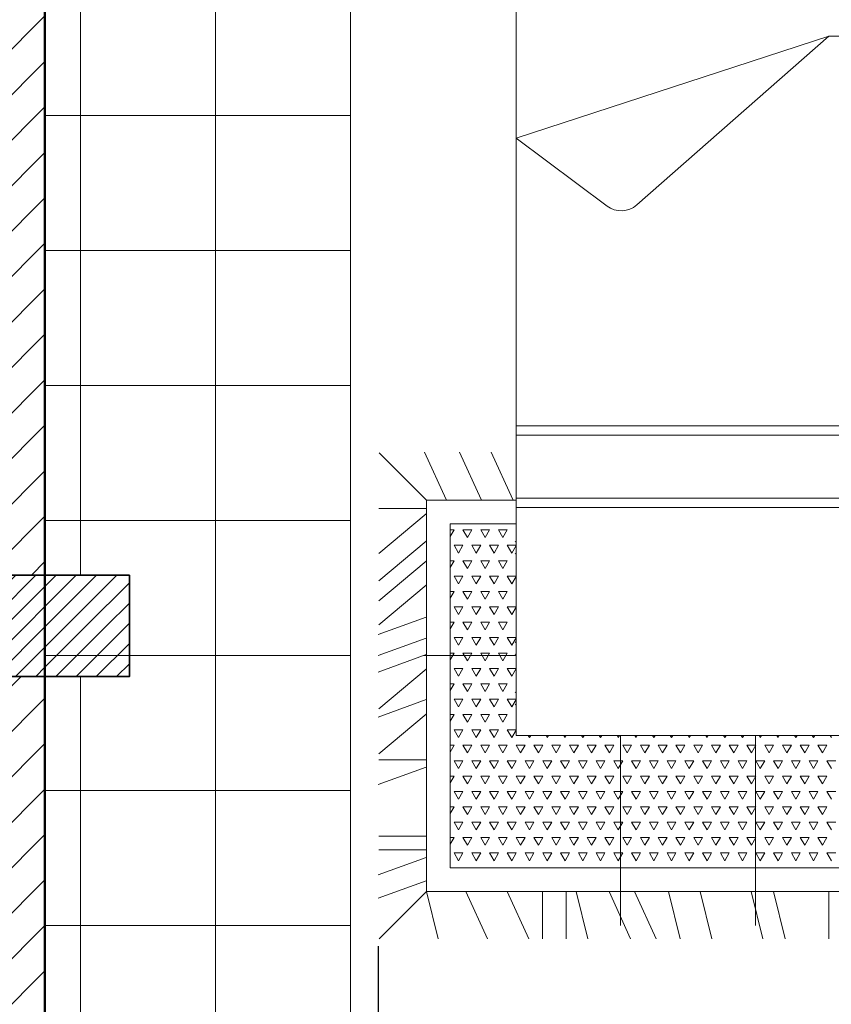
# Model space of a CAD drawing. Units: millimetres. Extents: x 225995 to 227247, y 225507 to 226008.
# Tile 19 of 23: x 227029 to 227101, y 225781 to 225868. Entities that reach past the tile are written whole.
import ezdxf

# ---------------------------------------------------------------- set-up
doc = ezdxf.new("R2010")
doc.units = ezdxf.units.MM
for name, color, linetype, lineweight in [('A-ANNO-DIMS', 2, 'Continuous', 18), ('A-COLS', 40, 'Continuous', 35), ('A-FLOR-PATT', 8, 'Continuous', 13), ('A-FURN', 9, 'Continuous', 18), ('A-WALL', 7, 'Continuous', 50), ('A-WALL-PATT', 8, 'Continuous', 13)]:
    doc.layers.add(name, color=color, linetype=linetype, lineweight=lineweight)
doc.styles.get("Standard").update_dxf_attribs({"font": 'arial.ttf'})
doc.dimstyles.new('ISO-25', dxfattribs={"dimtxt": 6, "dimasz": 2.5, "dimexe": 1.25, "dimexo": 0.625, "dimtad": 1, "dimdec": 0, "dimlunit": 3, "dimtxsty": 'Standard', "dimcen": 2.5, "dimadec": 0, "dimazin": 0, "dimtfac": 1, "dimtdec": 0, "dimtmove": 0, "dimatfit": 3, "dimfxl": 1, "dimarcsym": 0})
pattern_1 = [(45, (646.0463, 0.931), (-2.020557627, 2.020557627), [])]
pattern_2 = [(45, (646.0463, 119.0672), (-0.898025612, 0.898025612), [])]

# ---------------------------------------------------------------- blocks, each defined once
blk = doc.blocks.new('A$C6D2A2628')
for p, q in [((0.291, 0.4297), (0.291, 2.4297)), ((0.291, 1.6908), (0.9515, 1.9058)), ((0.9515, 1.9058), (0.5462, 1.5497)), ((0.9515, 1.9058), (1.1116, 1.9058)), ((0.4832, 1.5472), (0.291, 1.6908)), ((0.291, 1.0837), (1.791, 1.0837)), ((0.291, 1.0637), (1.791, 1.0637)), ((0.1019, 0.9267), (0.0019, 1.0267)), ((0.0977, 1.0278), (0.1431, 0.9278)), ((0.1716, 1.0278), (0.217, 0.9278)), ((0.2388, 1.0278), (0.2843, 0.9278)), ((0.291, 0.9267), (0.1019, 0.9267)), ((0.1019, 0.9267), (0.1019, 0.1)), ((0.291, 0.9307), (1.791, 0.9307)), ((0.0015, 0.9091), (0.1015, 0.9091)), ((0.0015, 0.8141), (0.1015, 0.8978)), ((0.291, 0.9107), (1.791, 0.9107)), ((0.291, 0.8767), (0.1519, 0.8767)), ((0.1519, 0.8767), (0.1519, 0.15)), ((0.1519, 0.8494), (0.1601, 0.8636)), ((0.1519, 0.8636), (0.1601, 0.8636)), ((0.1882, 0.8473), (0.1788, 0.8636)), ((0.1788, 0.8636), (0.1976, 0.8636)), ((0.1882, 0.8473), (0.1976, 0.8636)), ((0.2257, 0.8473), (0.2163, 0.8636)), ((0.2163, 0.8636), (0.2351, 0.8636)), ((0.2257, 0.8473), (0.2351, 0.8636)), ((0.2632, 0.8473), (0.2538, 0.8636)), ((0.2538, 0.8636), (0.2726, 0.8636)), ((0.2632, 0.8473), (0.2726, 0.8636)), ((0.0015, 0.7564), (0.1015, 0.84)), ((0.291, 0.8376), (0.2893, 0.8393)), ((0.1695, 0.8148), (0.1601, 0.8311)), ((0.1601, 0.8311), (0.1788, 0.8311)), ((0.1695, 0.8148), (0.1788, 0.8311)), ((0.207, 0.8148), (0.1976, 0.8311)), ((0.1976, 0.8311), (0.2163, 0.8311)), ((0.207, 0.8148), (0.2163, 0.8311)), ((0.2445, 0.8148), (0.2351, 0.8311)), ((0.2351, 0.8311), (0.2538, 0.8311)), ((0.2445, 0.8148), (0.2538, 0.8311)), ((0.282, 0.8148), (0.2726, 0.8311)), ((0.2726, 0.8311), (0.291, 0.8311)), ((0.282, 0.8148), (0.291, 0.8305)), ((0.291, 0.8144), (0.2893, 0.8128)), ((0.0015, 0.7139), (0.1015, 0.7975)), ((0.1519, 0.7844), (0.1601, 0.7986)), ((0.1519, 0.7986), (0.1601, 0.7986)), ((0.1882, 0.7824), (0.1788, 0.7986)), ((0.1788, 0.7986), (0.1976, 0.7986)), ((0.1882, 0.7824), (0.1976, 0.7986)), ((0.2257, 0.7824), (0.2163, 0.7986)), ((0.2163, 0.7986), (0.2351, 0.7986)), ((0.2257, 0.7824), (0.2351, 0.7986)), ((0.2632, 0.7824), (0.2538, 0.7986)), ((0.2538, 0.7986), (0.2726, 0.7986)), ((0.2632, 0.7824), (0.2726, 0.7986)), ((0.1695, 0.7499), (0.1601, 0.7661)), ((0.1601, 0.7661), (0.1788, 0.7661)), ((0.1695, 0.7499), (0.1788, 0.7661)), ((0.207, 0.7499), (0.1976, 0.7661)), ((0.1976, 0.7661), (0.2163, 0.7661)), ((0.207, 0.7499), (0.2163, 0.7661)), ((0.2445, 0.7499), (0.2351, 0.7661)), ((0.2351, 0.7661), (0.2538, 0.7661)), ((0.2445, 0.7499), (0.2538, 0.7661)), ((0.282, 0.7499), (0.2726, 0.7661)), ((0.2726, 0.7661), (0.291, 0.7661)), ((0.282, 0.7499), (0.291, 0.7655)), ((0.0015, 0.6633), (0.1015, 0.7469)), ((0.1519, 0.7195), (0.1601, 0.7337)), ((0.1519, 0.7337), (0.1601, 0.7337)), ((0.1882, 0.7174), (0.1788, 0.7337)), ((0.1788, 0.7337), (0.1976, 0.7337)), ((0.1882, 0.7174), (0.1976, 0.7337)), ((0.2257, 0.7174), (0.2163, 0.7337)), ((0.2163, 0.7337), (0.2351, 0.7337)), ((0.2257, 0.7174), (0.2351, 0.7337)), ((0.2632, 0.7174), (0.2538, 0.7337)), ((0.2538, 0.7337), (0.2726, 0.7337)), ((0.2632, 0.7174), (0.2726, 0.7337)), ((0.1695, 0.6849), (0.1601, 0.7012)), ((0.1601, 0.7012), (0.1788, 0.7012)), ((0.1695, 0.6849), (0.1788, 0.7012)), ((0.207, 0.6849), (0.1976, 0.7012)), ((0.1976, 0.7012), (0.2163, 0.7012)), ((0.207, 0.6849), (0.2163, 0.7012)), ((0.2445, 0.6849), (0.2351, 0.7012)), ((0.2351, 0.7012), (0.2538, 0.7012)), ((0.2445, 0.6849), (0.2538, 0.7012)), ((0.282, 0.6849), (0.2726, 0.7012)), ((0.2726, 0.7012), (0.291, 0.7012)), ((0.282, 0.6849), (0.291, 0.7006)), ((0, 0.6428), (0.1015, 0.6794)), ((0.1519, 0.6545), (0.1601, 0.6687)), ((0.1519, 0.6687), (0.1601, 0.6687)), ((0.1882, 0.6525), (0.1788, 0.6687)), ((0.1788, 0.6687), (0.1976, 0.6687)), ((0.1882, 0.6525), (0.1976, 0.6687)), ((0.2257, 0.6525), (0.2163, 0.6687)), ((0.2163, 0.6687), (0.2351, 0.6687)), ((0.2257, 0.6525), (0.2351, 0.6687)), ((0.2632, 0.6525), (0.2538, 0.6687)), ((0.2538, 0.6687), (0.2726, 0.6687)), ((0.2632, 0.6525), (0.2726, 0.6687)), ((0, 0.5984), (0.1015, 0.6351)), ((0.1695, 0.62), (0.1601, 0.6362)), ((0.1601, 0.6362), (0.1788, 0.6362)), ((0.1695, 0.62), (0.1788, 0.6362)), ((0.207, 0.62), (0.1976, 0.6362)), ((0.1976, 0.6362), (0.2163, 0.6362)), ((0.207, 0.62), (0.2163, 0.6362)), ((0.2445, 0.62), (0.2351, 0.6362)), ((0.2351, 0.6362), (0.2538, 0.6362)), ((0.2445, 0.62), (0.2538, 0.6362)), ((0.282, 0.62), (0.2726, 0.6362)), ((0.2726, 0.6362), (0.291, 0.6362)), ((0.282, 0.62), (0.291, 0.6356)), ((0.291, 0.6255), (0.2893, 0.6271)), ((0.1519, 0.5896), (0.1601, 0.6037)), ((0.1519, 0.6037), (0.1601, 0.6037)), ((0.1882, 0.5875), (0.1788, 0.6037)), ((0.1788, 0.6037), (0.1976, 0.6037)), ((0.1882, 0.5875), (0.1976, 0.6037)), ((0.2257, 0.5875), (0.2163, 0.6037)), ((0.2163, 0.6037), (0.2351, 0.6037)), ((0.2257, 0.5875), (0.2351, 0.6037)), ((0.2632, 0.5875), (0.2538, 0.6037)), ((0.2538, 0.6037), (0.2726, 0.6037)), ((0.2632, 0.5875), (0.2726, 0.6037)), ((0, 0.5636), (0.1015, 0.6003)), ((0.291, 0.6023), (0.2893, 0.6006)), ((0.0015, 0.4859), (0.1015, 0.5695)), ((0.1695, 0.555), (0.1601, 0.5713)), ((0.1601, 0.5713), (0.1788, 0.5713)), ((0.1695, 0.555), (0.1788, 0.5713)), ((0.207, 0.555), (0.1976, 0.5713)), ((0.1976, 0.5713), (0.2163, 0.5713)), ((0.207, 0.555), (0.2163, 0.5713)), ((0.2445, 0.555), (0.2351, 0.5713)), ((0.2351, 0.5713), (0.2538, 0.5713)), ((0.2445, 0.555), (0.2538, 0.5713)), ((0.282, 0.555), (0.2726, 0.5713)), ((0.2726, 0.5713), (0.291, 0.5713)), ((0.282, 0.555), (0.291, 0.5707)), ((0.1519, 0.5246), (0.1601, 0.5388)), ((0.1519, 0.5388), (0.1601, 0.5388)), ((0.1882, 0.5226), (0.1788, 0.5388)), ((0.1788, 0.5388), (0.1976, 0.5388)), ((0.1882, 0.5226), (0.1976, 0.5388)), ((0.2257, 0.5226), (0.2163, 0.5388)), ((0.2163, 0.5388), (0.2351, 0.5388)), ((0.2257, 0.5226), (0.2351, 0.5388)), ((0.2632, 0.5226), (0.2538, 0.5388)), ((0.2538, 0.5388), (0.2726, 0.5388)), ((0.2632, 0.5226), (0.2726, 0.5388)), ((0.291, 0.5194), (0.2893, 0.5211)), ((0, 0.4686), (0.1015, 0.5053)), ((0.1695, 0.4901), (0.1601, 0.5063)), ((0.1601, 0.5063), (0.1788, 0.5063)), ((0.1695, 0.4901), (0.1788, 0.5063)), ((0.207, 0.4901), (0.1976, 0.5063)), ((0.1976, 0.5063), (0.2163, 0.5063)), ((0.207, 0.4901), (0.2163, 0.5063)), ((0.2445, 0.4901), (0.2351, 0.5063)), ((0.2351, 0.5063), (0.2538, 0.5063)), ((0.2445, 0.4901), (0.2538, 0.5063)), ((0.282, 0.4901), (0.2726, 0.5063)), ((0.2726, 0.5063), (0.291, 0.5063)), ((0.282, 0.4901), (0.291, 0.5057)), ((0.291, 0.4962), (0.2893, 0.4946)), ((0.0015, 0.3909), (0.1015, 0.4745)), ((0.1519, 0.4597), (0.1601, 0.4738)), ((0.1519, 0.4738), (0.1601, 0.4738)), ((0.1882, 0.4576), (0.1788, 0.4738)), ((0.1788, 0.4738), (0.1976, 0.4738)), ((0.1882, 0.4576), (0.1976, 0.4738)), ((0.2257, 0.4576), (0.2163, 0.4738)), ((0.2163, 0.4738), (0.2351, 0.4738)), ((0.2257, 0.4576), (0.2351, 0.4738)), ((0.2632, 0.4576), (0.2538, 0.4738)), ((0.2538, 0.4738), (0.2726, 0.4738)), ((0.2632, 0.4576), (0.2726, 0.4738)), ((0.1695, 0.4251), (0.1601, 0.4414)), ((0.1601, 0.4414), (0.1788, 0.4414)), ((0.1695, 0.4251), (0.1788, 0.4414)), ((0.207, 0.4251), (0.1976, 0.4414)), ((0.1976, 0.4414), (0.2163, 0.4414)), ((0.207, 0.4251), (0.2163, 0.4414)), ((0.2445, 0.4251), (0.2351, 0.4414)), ((0.2351, 0.4414), (0.2538, 0.4414)), ((0.2445, 0.4251), (0.2538, 0.4414)), ((0.282, 0.4251), (0.2726, 0.4414)), ((0.2726, 0.4414), (0.291, 0.4414)), ((0.282, 0.4251), (0.291, 0.4408)), ((1.791, 0.4297), (0.291, 0.4297)), ((0.3195, 0.4251), (0.3168, 0.4297)), ((0.3195, 0.4251), (0.3221, 0.4297)), ((0.357, 0.4251), (0.3543, 0.4297)), ((0.357, 0.4251), (0.3596, 0.4297)), ((0.3945, 0.4251), (0.3918, 0.4297)), ((0.3945, 0.4251), (0.3971, 0.4297)), ((0.432, 0.4251), (0.4293, 0.4297)), ((0.432, 0.4251), (0.4346, 0.4297)), ((0.4695, 0.4251), (0.4668, 0.4297)), ((0.4695, 0.4251), (0.4721, 0.4297)), ((0.507, 0.4251), (0.5043, 0.4297)), ((0.507, 0.4251), (0.5096, 0.4297)), ((0.5445, 0.4251), (0.5418, 0.4297)), ((0.5445, 0.4251), (0.5471, 0.4297)), ((0.582, 0.4251), (0.5793, 0.4297)), ((0.582, 0.4251), (0.5846, 0.4297)), ((0.6195, 0.4251), (0.6168, 0.4297)), ((0.6195, 0.4251), (0.6221, 0.4297)), ((0.657, 0.4251), (0.6543, 0.4297)), ((0.657, 0.4251), (0.6596, 0.4297)), ((0.6945, 0.4251), (0.6918, 0.4297)), ((0.6945, 0.4251), (0.6971, 0.4297)), ((0.732, 0.4251), (0.7293, 0.4297)), ((0.732, 0.4251), (0.7346, 0.4297)), ((0.7695, 0.4251), (0.7668, 0.4297)), ((0.7695, 0.4251), (0.7721, 0.4297)), ((0.807, 0.4251), (0.8043, 0.4297)), ((0.807, 0.4251), (0.8096, 0.4297)), ((0.8445, 0.4251), (0.8418, 0.4297)), ((0.8445, 0.4251), (0.8471, 0.4297)), ((0.882, 0.4251), (0.8793, 0.4297)), ((0.882, 0.4251), (0.8846, 0.4297)), ((0.9195, 0.4251), (0.9168, 0.4297)), ((0.9195, 0.4251), (0.9221, 0.4297)), ((0.957, 0.4251), (0.9543, 0.4297)), ((0.1519, 0.3947), (0.1601, 0.4089)), ((0.1519, 0.4089), (0.1601, 0.4089)), ((0.1882, 0.3927), (0.1788, 0.4089)), ((0.1788, 0.4089), (0.1976, 0.4089)), ((0.1882, 0.3927), (0.1976, 0.4089)), ((0.2257, 0.3927), (0.2163, 0.4089)), ((0.2163, 0.4089), (0.2351, 0.4089)), ((0.2257, 0.3927), (0.2351, 0.4089)), ((0.2632, 0.3927), (0.2538, 0.4089)), ((0.2538, 0.4089), (0.2726, 0.4089)), ((0.2632, 0.3927), (0.2726, 0.4089)), ((0.3007, 0.3927), (0.2913, 0.4089)), ((0.2913, 0.4089), (0.3101, 0.4089)), ((0.3007, 0.3927), (0.3101, 0.4089)), ((0.3382, 0.3927), (0.3288, 0.4089)), ((0.3288, 0.4089), (0.3476, 0.4089)), ((0.3382, 0.3927), (0.3476, 0.4089)), ((0.3757, 0.3927), (0.3663, 0.4089)), ((0.3663, 0.4089), (0.3851, 0.4089)), ((0.3757, 0.3927), (0.3851, 0.4089)), ((0.4132, 0.3927), (0.4038, 0.4089)), ((0.4038, 0.4089), (0.4226, 0.4089)), ((0.4132, 0.3927), (0.4226, 0.4089)), ((0.4507, 0.3927), (0.4413, 0.4089)), ((0.4413, 0.4089), (0.4601, 0.4089)), ((0.4507, 0.3927), (0.4601, 0.4089)), ((0.4882, 0.3927), (0.4788, 0.4089)), ((0.4788, 0.4089), (0.4976, 0.4089)), ((0.4882, 0.3927), (0.4976, 0.4089)), ((0.5257, 0.3927), (0.5163, 0.4089)), ((0.5163, 0.4089), (0.5351, 0.4089)), ((0.5257, 0.3927), (0.5351, 0.4089)), ((0.5632, 0.3927), (0.5538, 0.4089)), ((0.5538, 0.4089), (0.5726, 0.4089)), ((0.5632, 0.3927), (0.5726, 0.4089)), ((0.6007, 0.3927), (0.5913, 0.4089)), ((0.5913, 0.4089), (0.6101, 0.4089)), ((0.6007, 0.3927), (0.6101, 0.4089)), ((0.6382, 0.3927), (0.6288, 0.4089)), ((0.6288, 0.4089), (0.6476, 0.4089)), ((0.6382, 0.3927), (0.6476, 0.4089)), ((0.6757, 0.3927), (0.6663, 0.4089)), ((0.6663, 0.4089), (0.6851, 0.4089)), ((0.6757, 0.3927), (0.6851, 0.4089)), ((0.7132, 0.3927), (0.7038, 0.4089)), ((0.7038, 0.4089), (0.7226, 0.4089)), ((0.7132, 0.3927), (0.7226, 0.4089)), ((0.7507, 0.3927), (0.7413, 0.4089)), ((0.7413, 0.4089), (0.7601, 0.4089)), ((0.7507, 0.3927), (0.7601, 0.4089)), ((0.7882, 0.3927), (0.7788, 0.4089)), ((0.7788, 0.4089), (0.7976, 0.4089)), ((0.7882, 0.3927), (0.7976, 0.4089)), ((0.8257, 0.3927), (0.8163, 0.4089)), ((0.8163, 0.4089), (0.8351, 0.4089)), ((0.8257, 0.3927), (0.8351, 0.4089)), ((0.8632, 0.3927), (0.8538, 0.4089)), ((0.8538, 0.4089), (0.8726, 0.4089)), ((0.8632, 0.3927), (0.8726, 0.4089)), ((0.9007, 0.3927), (0.8913, 0.4089)), ((0.8913, 0.4089), (0.9101, 0.4089)), ((0.9007, 0.3927), (0.9101, 0.4089)), ((0.9382, 0.3927), (0.9288, 0.4089)), ((0.9288, 0.4089), (0.9476, 0.4089)), ((0.9382, 0.3927), (0.9476, 0.4089)), ((0.0015, 0.3783), (0.1015, 0.3783)), ((0.1695, 0.3602), (0.1601, 0.3764)), ((0.1601, 0.3764), (0.1788, 0.3764)), ((0.1695, 0.3602), (0.1788, 0.3764)), ((0.207, 0.3602), (0.1976, 0.3764)), ((0.1976, 0.3764), (0.2163, 0.3764)), ((0.207, 0.3602), (0.2163, 0.3764)), ((0.2445, 0.3602), (0.2351, 0.3764)), ((0.2351, 0.3764), (0.2538, 0.3764)), ((0.2445, 0.3602), (0.2538, 0.3764)), ((0.282, 0.3602), (0.2726, 0.3764)), ((0.2726, 0.3764), (0.2913, 0.3764)), ((0.282, 0.3602), (0.2913, 0.3764)), ((0.3195, 0.3602), (0.3101, 0.3764)), ((0.3101, 0.3764), (0.3288, 0.3764)), ((0.3195, 0.3602), (0.3288, 0.3764)), ((0.357, 0.3602), (0.3476, 0.3764)), ((0.3476, 0.3764), (0.3663, 0.3764)), ((0.357, 0.3602), (0.3663, 0.3764)), ((0.3945, 0.3602), (0.3851, 0.3764)), ((0.3851, 0.3764), (0.4038, 0.3764)), ((0.3945, 0.3602), (0.4038, 0.3764)), ((0.432, 0.3602), (0.4226, 0.3764)), ((0.4226, 0.3764), (0.4413, 0.3764)), ((0.432, 0.3602), (0.4413, 0.3764)), ((0.4695, 0.3602), (0.4601, 0.3764)), ((0.4601, 0.3764), (0.4788, 0.3764)), ((0.4695, 0.3602), (0.4788, 0.3764)), ((0.507, 0.3602), (0.4976, 0.3764)), ((0.4976, 0.3764), (0.5163, 0.3764)), ((0.507, 0.3602), (0.5163, 0.3764)), ((0.5445, 0.3602), (0.5351, 0.3764)), ((0.5351, 0.3764), (0.5538, 0.3764)), ((0.5445, 0.3602), (0.5538, 0.3764)), ((0.582, 0.3602), (0.5726, 0.3764)), ((0.5726, 0.3764), (0.5913, 0.3764)), ((0.582, 0.3602), (0.5913, 0.3764)), ((0.6195, 0.3602), (0.6101, 0.3764)), ((0.6101, 0.3764), (0.6288, 0.3764)), ((0.6195, 0.3602), (0.6288, 0.3764)), ((0.657, 0.3602), (0.6476, 0.3764)), ((0.6476, 0.3764), (0.6663, 0.3764)), ((0.657, 0.3602), (0.6663, 0.3764)), ((0.6945, 0.3602), (0.6851, 0.3764)), ((0.6851, 0.3764), (0.7038, 0.3764)), ((0.6945, 0.3602), (0.7038, 0.3764)), ((0.732, 0.3602), (0.7226, 0.3764)), ((0.7226, 0.3764), (0.7413, 0.3764)), ((0.732, 0.3602), (0.7413, 0.3764)), ((0.7695, 0.3602), (0.7601, 0.3764)), ((0.7601, 0.3764), (0.7788, 0.3764)), ((0.7695, 0.3602), (0.7788, 0.3764)), ((0.807, 0.3602), (0.7976, 0.3764)), ((0.7976, 0.3764), (0.8163, 0.3764)), ((0.807, 0.3602), (0.8163, 0.3764)), ((0.8445, 0.3602), (0.8351, 0.3764)), ((0.8351, 0.3764), (0.8538, 0.3764)), ((0.8445, 0.3602), (0.8538, 0.3764)), ((0.882, 0.3602), (0.8726, 0.3764)), ((0.8726, 0.3764), (0.8913, 0.3764)), ((0.882, 0.3602), (0.8913, 0.3764)), ((0.9195, 0.3602), (0.9101, 0.3764)), ((0.9101, 0.3764), (0.9288, 0.3764)), ((0.9195, 0.3602), (0.9288, 0.3764)), ((0.957, 0.3602), (0.9476, 0.3764)), ((0.9476, 0.3764), (0.9663, 0.3764)), ((0, 0.3261), (0.1015, 0.3628)), ((0.1519, 0.3298), (0.1601, 0.3439)), ((0.1519, 0.3439), (0.1601, 0.3439)), ((0.1882, 0.3277), (0.1788, 0.3439)), ((0.1788, 0.3439), (0.1976, 0.3439)), ((0.1882, 0.3277), (0.1976, 0.3439)), ((0.2257, 0.3277), (0.2163, 0.3439)), ((0.2163, 0.3439), (0.2351, 0.3439)), ((0.2257, 0.3277), (0.2351, 0.3439)), ((0.2632, 0.3277), (0.2538, 0.3439)), ((0.2538, 0.3439), (0.2726, 0.3439)), ((0.2632, 0.3277), (0.2726, 0.3439)), ((0.3007, 0.3277), (0.2913, 0.3439)), ((0.2913, 0.3439), (0.3101, 0.3439)), ((0.3007, 0.3277), (0.3101, 0.3439)), ((0.3382, 0.3277), (0.3288, 0.3439)), ((0.3288, 0.3439), (0.3476, 0.3439)), ((0.3382, 0.3277), (0.3476, 0.3439)), ((0.3757, 0.3277), (0.3663, 0.3439)), ((0.3663, 0.3439), (0.3851, 0.3439)), ((0.3757, 0.3277), (0.3851, 0.3439)), ((0.4132, 0.3277), (0.4038, 0.3439)), ((0.4038, 0.3439), (0.4226, 0.3439)), ((0.4132, 0.3277), (0.4226, 0.3439)), ((0.4507, 0.3277), (0.4413, 0.3439)), ((0.4413, 0.3439), (0.4601, 0.3439)), ((0.4507, 0.3277), (0.4601, 0.3439)), ((0.4882, 0.3277), (0.4788, 0.3439)), ((0.4788, 0.3439), (0.4976, 0.3439)), ((0.4882, 0.3277), (0.4976, 0.3439)), ((0.5257, 0.3277), (0.5163, 0.3439)), ((0.5163, 0.3439), (0.5351, 0.3439)), ((0.5257, 0.3277), (0.5351, 0.3439)), ((0.5632, 0.3277), (0.5538, 0.3439)), ((0.5538, 0.3439), (0.5726, 0.3439)), ((0.5632, 0.3277), (0.5726, 0.3439)), ((0.6007, 0.3277), (0.5913, 0.3439)), ((0.5913, 0.3439), (0.6101, 0.3439)), ((0.6007, 0.3277), (0.6101, 0.3439)), ((0.6382, 0.3277), (0.6288, 0.3439)), ((0.6288, 0.3439), (0.6476, 0.3439)), ((0.6382, 0.3277), (0.6476, 0.3439)), ((0.6757, 0.3277), (0.6663, 0.3439)), ((0.6663, 0.3439), (0.6851, 0.3439)), ((0.6757, 0.3277), (0.6851, 0.3439)), ((0.7132, 0.3277), (0.7038, 0.3439)), ((0.7038, 0.3439), (0.7226, 0.3439)), ((0.7132, 0.3277), (0.7226, 0.3439)), ((0.7507, 0.3277), (0.7413, 0.3439)), ((0.7413, 0.3439), (0.7601, 0.3439)), ((0.7507, 0.3277), (0.7601, 0.3439)), ((0.7882, 0.3277), (0.7788, 0.3439)), ((0.7788, 0.3439), (0.7976, 0.3439)), ((0.7882, 0.3277), (0.7976, 0.3439)), ((0.8257, 0.3277), (0.8163, 0.3439)), ((0.8163, 0.3439), (0.8351, 0.3439)), ((0.8257, 0.3277), (0.8351, 0.3439)), ((0.8632, 0.3277), (0.8538, 0.3439)), ((0.8538, 0.3439), (0.8726, 0.3439)), ((0.8632, 0.3277), (0.8726, 0.3439)), ((0.9007, 0.3277), (0.8913, 0.3439)), ((0.8913, 0.3439), (0.9101, 0.3439)), ((0.9007, 0.3277), (0.9101, 0.3439)), ((0.9382, 0.3277), (0.9288, 0.3439)), ((0.9288, 0.3439), (0.9476, 0.3439)), ((0.9382, 0.3277), (0.9476, 0.3439)), ((0.1695, 0.2952), (0.1601, 0.3115)), ((0.1601, 0.3115), (0.1788, 0.3115)), ((0.1695, 0.2952), (0.1788, 0.3115)), ((0.207, 0.2952), (0.1976, 0.3115)), ((0.1976, 0.3115), (0.2163, 0.3115)), ((0.207, 0.2952), (0.2163, 0.3115)), ((0.2445, 0.2952), (0.2351, 0.3115)), ((0.2351, 0.3115), (0.2538, 0.3115)), ((0.2445, 0.2952), (0.2538, 0.3115)), ((0.282, 0.2952), (0.2726, 0.3115)), ((0.2726, 0.3115), (0.2913, 0.3115)), ((0.282, 0.2952), (0.2913, 0.3115)), ((0.3195, 0.2952), (0.3101, 0.3115)), ((0.3101, 0.3115), (0.3288, 0.3115)), ((0.3195, 0.2952), (0.3288, 0.3115)), ((0.357, 0.2952), (0.3476, 0.3115)), ((0.3476, 0.3115), (0.3663, 0.3115)), ((0.357, 0.2952), (0.3663, 0.3115)), ((0.3945, 0.2952), (0.3851, 0.3115)), ((0.3851, 0.3115), (0.4038, 0.3115)), ((0.3945, 0.2952), (0.4038, 0.3115)), ((0.432, 0.2952), (0.4226, 0.3115)), ((0.4226, 0.3115), (0.4413, 0.3115)), ((0.432, 0.2952), (0.4413, 0.3115)), ((0.4695, 0.2952), (0.4601, 0.3115)), ((0.4601, 0.3115), (0.4788, 0.3115)), ((0.4695, 0.2952), (0.4788, 0.3115)), ((0.507, 0.2952), (0.4976, 0.3115)), ((0.4976, 0.3115), (0.5163, 0.3115)), ((0.507, 0.2952), (0.5163, 0.3115)), ((0.5445, 0.2952), (0.5351, 0.3115)), ((0.5351, 0.3115), (0.5538, 0.3115)), ((0.5445, 0.2952), (0.5538, 0.3115)), ((0.582, 0.2952), (0.5726, 0.3115)), ((0.5726, 0.3115), (0.5913, 0.3115)), ((0.582, 0.2952), (0.5913, 0.3115)), ((0.6195, 0.2952), (0.6101, 0.3115)), ((0.6101, 0.3115), (0.6288, 0.3115)), ((0.6195, 0.2952), (0.6288, 0.3115)), ((0.657, 0.2952), (0.6476, 0.3115)), ((0.6476, 0.3115), (0.6663, 0.3115)), ((0.657, 0.2952), (0.6663, 0.3115)), ((0.6945, 0.2952), (0.6851, 0.3115)), ((0.6851, 0.3115), (0.7038, 0.3115)), ((0.6945, 0.2952), (0.7038, 0.3115)), ((0.732, 0.2952), (0.7226, 0.3115)), ((0.7226, 0.3115), (0.7413, 0.3115)), ((0.732, 0.2952), (0.7413, 0.3115)), ((0.7695, 0.2952), (0.7601, 0.3115)), ((0.7601, 0.3115), (0.7788, 0.3115)), ((0.7695, 0.2952), (0.7788, 0.3115)), ((0.807, 0.2952), (0.7976, 0.3115)), ((0.7976, 0.3115), (0.8163, 0.3115)), ((0.807, 0.2952), (0.8163, 0.3115)), ((0.8445, 0.2952), (0.8351, 0.3115)), ((0.8351, 0.3115), (0.8538, 0.3115)), ((0.8445, 0.2952), (0.8538, 0.3115)), ((0.882, 0.2952), (0.8726, 0.3115)), ((0.8726, 0.3115), (0.8913, 0.3115)), ((0.882, 0.2952), (0.8913, 0.3115)), ((0.9195, 0.2952), (0.9101, 0.3115)), ((0.9101, 0.3115), (0.9288, 0.3115)), ((0.9195, 0.2952), (0.9288, 0.3115)), ((0.957, 0.2952), (0.9476, 0.3115)), ((0.9476, 0.3115), (0.9663, 0.3115)), ((0.1519, 0.2648), (0.1601, 0.279)), ((0.1519, 0.279), (0.1601, 0.279)), ((0.1882, 0.2628), (0.1788, 0.279)), ((0.1788, 0.279), (0.1976, 0.279)), ((0.1882, 0.2628), (0.1976, 0.279)), ((0.2257, 0.2628), (0.2163, 0.279)), ((0.2163, 0.279), (0.2351, 0.279)), ((0.2257, 0.2628), (0.2351, 0.279)), ((0.2632, 0.2628), (0.2538, 0.279)), ((0.2538, 0.279), (0.2726, 0.279)), ((0.2632, 0.2628), (0.2726, 0.279)), ((0.3007, 0.2628), (0.2913, 0.279)), ((0.2913, 0.279), (0.3101, 0.279)), ((0.3007, 0.2628), (0.3101, 0.279)), ((0.3382, 0.2628), (0.3288, 0.279)), ((0.3288, 0.279), (0.3476, 0.279)), ((0.3382, 0.2628), (0.3476, 0.279)), ((0.3757, 0.2628), (0.3663, 0.279)), ((0.3663, 0.279), (0.3851, 0.279)), ((0.3757, 0.2628), (0.3851, 0.279)), ((0.4132, 0.2628), (0.4038, 0.279)), ((0.4038, 0.279), (0.4226, 0.279)), ((0.4132, 0.2628), (0.4226, 0.279)), ((0.4507, 0.2628), (0.4413, 0.279)), ((0.4413, 0.279), (0.4601, 0.279)), ((0.4507, 0.2628), (0.4601, 0.279)), ((0.4882, 0.2628), (0.4788, 0.279)), ((0.4788, 0.279), (0.4976, 0.279)), ((0.4882, 0.2628), (0.4976, 0.279)), ((0.5257, 0.2628), (0.5163, 0.279)), ((0.5163, 0.279), (0.5351, 0.279)), ((0.5257, 0.2628), (0.5351, 0.279)), ((0.5632, 0.2628), (0.5538, 0.279)), ((0.5538, 0.279), (0.5726, 0.279)), ((0.5632, 0.2628), (0.5726, 0.279)), ((0.6007, 0.2628), (0.5913, 0.279)), ((0.5913, 0.279), (0.6101, 0.279)), ((0.6007, 0.2628), (0.6101, 0.279)), ((0.6382, 0.2628), (0.6288, 0.279)), ((0.6288, 0.279), (0.6476, 0.279)), ((0.6382, 0.2628), (0.6476, 0.279)), ((0.6757, 0.2628), (0.6663, 0.279)), ((0.6663, 0.279), (0.6851, 0.279)), ((0.6757, 0.2628), (0.6851, 0.279)), ((0.7132, 0.2628), (0.7038, 0.279)), ((0.7038, 0.279), (0.7226, 0.279)), ((0.7132, 0.2628), (0.7226, 0.279)), ((0.7507, 0.2628), (0.7413, 0.279)), ((0.7413, 0.279), (0.7601, 0.279)), ((0.7507, 0.2628), (0.7601, 0.279)), ((0.7882, 0.2628), (0.7788, 0.279)), ((0.7788, 0.279), (0.7976, 0.279)), ((0.7882, 0.2628), (0.7976, 0.279)), ((0.8257, 0.2628), (0.8163, 0.279)), ((0.8163, 0.279), (0.8351, 0.279)), ((0.8257, 0.2628), (0.8351, 0.279)), ((0.8632, 0.2628), (0.8538, 0.279)), ((0.8538, 0.279), (0.8726, 0.279)), ((0.8632, 0.2628), (0.8726, 0.279)), ((0.9007, 0.2628), (0.8913, 0.279)), ((0.8913, 0.279), (0.9101, 0.279)), ((0.9007, 0.2628), (0.9101, 0.279)), ((0.9382, 0.2628), (0.9288, 0.279)), ((0.9288, 0.279), (0.9476, 0.279)), ((0.9382, 0.2628), (0.9476, 0.279)), ((0.1695, 0.2303), (0.1601, 0.2465)), ((0.1601, 0.2465), (0.1788, 0.2465)), ((0.1695, 0.2303), (0.1788, 0.2465)), ((0.207, 0.2303), (0.1976, 0.2465)), ((0.1976, 0.2465), (0.2163, 0.2465)), ((0.207, 0.2303), (0.2163, 0.2465)), ((0.2445, 0.2303), (0.2351, 0.2465)), ((0.2351, 0.2465), (0.2538, 0.2465)), ((0.2445, 0.2303), (0.2538, 0.2465)), ((0.282, 0.2303), (0.2726, 0.2465)), ((0.2726, 0.2465), (0.2913, 0.2465)), ((0.282, 0.2303), (0.2913, 0.2465)), ((0.3195, 0.2303), (0.3101, 0.2465)), ((0.3101, 0.2465), (0.3288, 0.2465)), ((0.3195, 0.2303), (0.3288, 0.2465)), ((0.357, 0.2303), (0.3476, 0.2465)), ((0.3476, 0.2465), (0.3663, 0.2465)), ((0.357, 0.2303), (0.3663, 0.2465)), ((0.3945, 0.2303), (0.3851, 0.2465)), ((0.3851, 0.2465), (0.4038, 0.2465)), ((0.3945, 0.2303), (0.4038, 0.2465)), ((0.432, 0.2303), (0.4226, 0.2465)), ((0.4226, 0.2465), (0.4413, 0.2465)), ((0.432, 0.2303), (0.4413, 0.2465)), ((0.4695, 0.2303), (0.4601, 0.2465)), ((0.4601, 0.2465), (0.4788, 0.2465)), ((0.4695, 0.2303), (0.4788, 0.2465)), ((0.507, 0.2303), (0.4976, 0.2465)), ((0.4976, 0.2465), (0.5163, 0.2465)), ((0.507, 0.2303), (0.5163, 0.2465)), ((0.5445, 0.2303), (0.5351, 0.2465)), ((0.5351, 0.2465), (0.5538, 0.2465)), ((0.5445, 0.2303), (0.5538, 0.2465)), ((0.582, 0.2303), (0.5726, 0.2465)), ((0.5726, 0.2465), (0.5913, 0.2465)), ((0.582, 0.2303), (0.5913, 0.2465)), ((0.6195, 0.2303), (0.6101, 0.2465)), ((0.6101, 0.2465), (0.6288, 0.2465)), ((0.6195, 0.2303), (0.6288, 0.2465)), ((0.657, 0.2303), (0.6476, 0.2465)), ((0.6476, 0.2465), (0.6663, 0.2465)), ((0.657, 0.2303), (0.6663, 0.2465)), ((0.6945, 0.2303), (0.6851, 0.2465)), ((0.6851, 0.2465), (0.7038, 0.2465)), ((0.6945, 0.2303), (0.7038, 0.2465)), ((0.732, 0.2303), (0.7226, 0.2465)), ((0.7226, 0.2465), (0.7413, 0.2465)), ((0.732, 0.2303), (0.7413, 0.2465)), ((0.7695, 0.2303), (0.7601, 0.2465)), ((0.7601, 0.2465), (0.7788, 0.2465)), ((0.7695, 0.2303), (0.7788, 0.2465)), ((0.807, 0.2303), (0.7976, 0.2465)), ((0.7976, 0.2465), (0.8163, 0.2465)), ((0.807, 0.2303), (0.8163, 0.2465)), ((0.8445, 0.2303), (0.8351, 0.2465)), ((0.8351, 0.2465), (0.8538, 0.2465)), ((0.8445, 0.2303), (0.8538, 0.2465)), ((0.882, 0.2303), (0.8726, 0.2465)), ((0.8726, 0.2465), (0.8913, 0.2465)), ((0.882, 0.2303), (0.8913, 0.2465)), ((0.9195, 0.2303), (0.9101, 0.2465)), ((0.9101, 0.2465), (0.9288, 0.2465)), ((0.9195, 0.2303), (0.9288, 0.2465)), ((0.957, 0.2303), (0.9476, 0.2465)), ((0.9476, 0.2465), (0.9663, 0.2465)), ((0.0015, 0.2173), (0.1015, 0.2173)), ((0.1519, 0.1999), (0.1601, 0.214)), ((0.1519, 0.214), (0.1601, 0.214)), ((0.1882, 0.1978), (0.1788, 0.214)), ((0.1788, 0.214), (0.1976, 0.214)), ((0.1882, 0.1978), (0.1976, 0.214)), ((0.2257, 0.1978), (0.2163, 0.214)), ((0.2163, 0.214), (0.2351, 0.214)), ((0.2257, 0.1978), (0.2351, 0.214)), ((0.2632, 0.1978), (0.2538, 0.214)), ((0.2538, 0.214), (0.2726, 0.214)), ((0.2632, 0.1978), (0.2726, 0.214)), ((0.3007, 0.1978), (0.2913, 0.214)), ((0.2913, 0.214), (0.3101, 0.214)), ((0.3007, 0.1978), (0.3101, 0.214)), ((0.3382, 0.1978), (0.3288, 0.214)), ((0.3288, 0.214), (0.3476, 0.214)), ((0.3382, 0.1978), (0.3476, 0.214)), ((0.3757, 0.1978), (0.3663, 0.214)), ((0.3663, 0.214), (0.3851, 0.214)), ((0.3757, 0.1978), (0.3851, 0.214)), ((0.4132, 0.1978), (0.4038, 0.214)), ((0.4038, 0.214), (0.4226, 0.214)), ((0.4132, 0.1978), (0.4226, 0.214)), ((0.4507, 0.1978), (0.4413, 0.214)), ((0.4413, 0.214), (0.4601, 0.214)), ((0.4507, 0.1978), (0.4601, 0.214)), ((0.4882, 0.1978), (0.4788, 0.214)), ((0.4788, 0.214), (0.4976, 0.214)), ((0.4882, 0.1978), (0.4976, 0.214)), ((0.5257, 0.1978), (0.5163, 0.214)), ((0.5163, 0.214), (0.5351, 0.214)), ((0.5257, 0.1978), (0.5351, 0.214)), ((0.5632, 0.1978), (0.5538, 0.214)), ((0.5538, 0.214), (0.5726, 0.214)), ((0.5632, 0.1978), (0.5726, 0.214)), ((0.6007, 0.1978), (0.5913, 0.214)), ((0.5913, 0.214), (0.6101, 0.214)), ((0.6007, 0.1978), (0.6101, 0.214)), ((0.6382, 0.1978), (0.6288, 0.214)), ((0.6288, 0.214), (0.6476, 0.214)), ((0.6382, 0.1978), (0.6476, 0.214)), ((0.6757, 0.1978), (0.6663, 0.214)), ((0.6663, 0.214), (0.6851, 0.214)), ((0.6757, 0.1978), (0.6851, 0.214)), ((0.7132, 0.1978), (0.7038, 0.214)), ((0.7038, 0.214), (0.7226, 0.214)), ((0.7132, 0.1978), (0.7226, 0.214)), ((0.7507, 0.1978), (0.7413, 0.214)), ((0.7413, 0.214), (0.7601, 0.214)), ((0.7507, 0.1978), (0.7601, 0.214)), ((0.7882, 0.1978), (0.7788, 0.214)), ((0.7788, 0.214), (0.7976, 0.214)), ((0.7882, 0.1978), (0.7976, 0.214)), ((0.8257, 0.1978), (0.8163, 0.214)), ((0.8163, 0.214), (0.8351, 0.214)), ((0.8257, 0.1978), (0.8351, 0.214)), ((0.8632, 0.1978), (0.8538, 0.214)), ((0.8538, 0.214), (0.8726, 0.214)), ((0.8632, 0.1978), (0.8726, 0.214)), ((0.9007, 0.1978), (0.8913, 0.214)), ((0.8913, 0.214), (0.9101, 0.214)), ((0.9007, 0.1978), (0.9101, 0.214)), ((0.9382, 0.1978), (0.9288, 0.214)), ((0.9288, 0.214), (0.9476, 0.214)), ((0.9382, 0.1978), (0.9476, 0.214)), ((0.0015, 0.1884), (0.1015, 0.1884)), ((0, 0.1355), (0.1015, 0.1722)), ((0.1695, 0.1653), (0.1601, 0.1816)), ((0.1601, 0.1816), (0.1788, 0.1816)), ((0.1695, 0.1653), (0.1788, 0.1816)), ((0.207, 0.1653), (0.1976, 0.1816)), ((0.1976, 0.1816), (0.2163, 0.1816)), ((0.207, 0.1653), (0.2163, 0.1816)), ((0.2445, 0.1653), (0.2351, 0.1816)), ((0.2351, 0.1816), (0.2538, 0.1816)), ((0.2445, 0.1653), (0.2538, 0.1816)), ((0.282, 0.1653), (0.2726, 0.1816)), ((0.2726, 0.1816), (0.2913, 0.1816)), ((0.282, 0.1653), (0.2913, 0.1816)), ((0.3195, 0.1653), (0.3101, 0.1816)), ((0.3101, 0.1816), (0.3288, 0.1816)), ((0.3195, 0.1653), (0.3288, 0.1816)), ((0.357, 0.1653), (0.3476, 0.1816)), ((0.3476, 0.1816), (0.3663, 0.1816)), ((0.357, 0.1653), (0.3663, 0.1816)), ((0.3945, 0.1653), (0.3851, 0.1816)), ((0.3851, 0.1816), (0.4038, 0.1816)), ((0.3945, 0.1653), (0.4038, 0.1816)), ((0.432, 0.1653), (0.4226, 0.1816)), ((0.4226, 0.1816), (0.4413, 0.1816)), ((0.432, 0.1653), (0.4413, 0.1816)), ((0.4695, 0.1653), (0.4601, 0.1816)), ((0.4601, 0.1816), (0.4788, 0.1816)), ((0.4695, 0.1653), (0.4788, 0.1816)), ((0.507, 0.1653), (0.4976, 0.1816)), ((0.4976, 0.1816), (0.5163, 0.1816)), ((0.507, 0.1653), (0.5163, 0.1816)), ((0.5445, 0.1653), (0.5351, 0.1816)), ((0.5351, 0.1816), (0.5538, 0.1816)), ((0.5445, 0.1653), (0.5538, 0.1816)), ((0.582, 0.1653), (0.5726, 0.1816)), ((0.5726, 0.1816), (0.5913, 0.1816)), ((0.582, 0.1653), (0.5913, 0.1816)), ((0.6195, 0.1653), (0.6101, 0.1816)), ((0.6101, 0.1816), (0.6288, 0.1816)), ((0.6195, 0.1653), (0.6288, 0.1816)), ((0.657, 0.1653), (0.6476, 0.1816)), ((0.6476, 0.1816), (0.6663, 0.1816)), ((0.657, 0.1653), (0.6663, 0.1816)), ((0.6945, 0.1653), (0.6851, 0.1816)), ((0.6851, 0.1816), (0.7038, 0.1816)), ((0.6945, 0.1653), (0.7038, 0.1816)), ((0.732, 0.1653), (0.7226, 0.1816)), ((0.7226, 0.1816), (0.7413, 0.1816)), ((0.732, 0.1653), (0.7413, 0.1816)), ((0.7695, 0.1653), (0.7601, 0.1816)), ((0.7601, 0.1816), (0.7788, 0.1816)), ((0.7695, 0.1653), (0.7788, 0.1816)), ((0.807, 0.1653), (0.7976, 0.1816)), ((0.7976, 0.1816), (0.8163, 0.1816)), ((0.807, 0.1653), (0.8163, 0.1816)), ((0.8445, 0.1653), (0.8351, 0.1816)), ((0.8351, 0.1816), (0.8538, 0.1816)), ((0.8445, 0.1653), (0.8538, 0.1816)), ((0.882, 0.1653), (0.8726, 0.1816)), ((0.8726, 0.1816), (0.8913, 0.1816)), ((0.882, 0.1653), (0.8913, 0.1816)), ((0.9195, 0.1653), (0.9101, 0.1816)), ((0.9101, 0.1816), (0.9288, 0.1816)), ((0.9195, 0.1653), (0.9288, 0.1816)), ((0.957, 0.1653), (0.9476, 0.1816)), ((0.9476, 0.1816), (0.9663, 0.1816)), ((0.1519, 0.15), (1.9432, 0.15)), ((0, 0.0863), (0.1015, 0.1229)), ((0.1019, 0.1), (0.0019, 0)), ((0.1019, 0.1), (1.9932, 0.1)), ((0.1019, 0.1), (0.1266, 0)), ((0.1851, 0.1), (0.2305, 0)), ((0.2725, 0.1), (0.3179, 0)), ((0.3469, 0.1), (0.3469, 0)), ((0.3969, 0.1), (0.3969, 0)), ((0.4179, 0.1), (0.4426, 0)), ((0.4876, 0.1), (0.533, 0)), ((0.5414, 0.1), (0.5868, 0)), ((0.6128, 0.1), (0.6376, 0)), ((0.6801, 0.1), (0.7048, 0)), ((0.7876, 0.1), (0.8124, 0)), ((0.8347, 0.1), (0.8594, 0)), ((0.952, 0.1), (0.952, 0))]:
    blk.add_line(p, q)
blk.add_arc((0.5131, 1.5873), 0.05, 233.2421, 311.3042)
blk = doc.blocks.new('*D80')
at = {"layer": 'A-ANNO-DIMS', "color": 0, "lineweight": -2, "transparency": 16777216}
for p, q in [((227060.554, 225785.895), (227060.554, 225769.929)), ((227148.657, 225785.895), (227148.657, 225769.929)), ((227063.054, 225771.179), (227146.157, 225771.179))]:
    blk.add_line(p, q, dxfattribs=at)
at = {"layer": 'A-ANNO-DIMS', "color": 0, "transparency": 16777216}
for points in [[(227063.054, 225771.596), (227063.054, 225770.762), (227060.554, 225771.179)], [(227146.157, 225771.596), (227146.157, 225770.762), (227148.657, 225771.179)]]:
    blk.add_solid(points, dxfattribs=at)
at = {"layer": 'Defpoints', "color": 0, "transparency": 16777216}
for p in [(227060.554, 225786.52), (227148.657, 225786.52), (227148.657, 225771.179)]:
    blk.add_point(p, dxfattribs=at)
at = {"layer": 'A-ANNO-DIMS', "color": 0, "transparency": 16777216, "insert": (227104.605, 225774.806), "char_height": 6, "attachment_point": 5}
blk.add_mtext('7\'-4" TYP.', dxfattribs=at)

msp = doc.modelspace()

# ---------------------------------------------------------------- hatches: boundary and pattern name
at = {"layer": 'A-WALL-PATT'}
h = msp.add_hatch(dxfattribs=at)
h.set_pattern_fill('ANSI31', color=256, scale=0.9)
h.set_pattern_definition(pattern_1)
h.paths.add_polyline_path([(227030.923, 225925.705), (227026.423, 225925.705), (227026.423, 225818.841), (227030.923, 225818.841)])
h = msp.add_hatch(dxfattribs=at)
h.set_pattern_fill('ANSI31', color=256, scale=0.4)
h.set_pattern_definition(pattern_2)
h.paths.add_polyline_path([(227030.923, 225818.841), (227026.423, 225818.841), (227026.423, 225814.341), (227030.923, 225814.341)])
h = msp.add_hatch(dxfattribs=at)
h.set_pattern_fill('ANSI31', color=256, scale=0.4)
h.set_pattern_definition(pattern_2)
h.paths.add_polyline_path([(227038.423, 225818.841), (227030.923, 225818.841), (227030.923, 225814.341), (227038.423, 225814.341)])
h = msp.add_hatch(dxfattribs=at)
h.set_pattern_fill('ANSI31', color=256, scale=0.4)
h.set_pattern_definition(pattern_2)
h.paths.add_polyline_path([(227030.923, 225814.341), (227026.423, 225814.341), (227026.423, 225809.841), (227030.923, 225809.841)])
h = msp.add_hatch(dxfattribs=at)
h.set_pattern_fill('ANSI31', color=256, scale=0.4)
h.set_pattern_definition(pattern_2)
h.paths.add_polyline_path([(227038.423, 225814.341), (227030.923, 225814.341), (227030.923, 225809.841), (227038.423, 225809.841)])
h = msp.add_hatch(dxfattribs=at)
h.set_pattern_fill('ANSI31', color=256, scale=0.9)
h.set_pattern_definition(pattern_1)
h.paths.add_polyline_path([(227030.923, 225809.841), (227026.423, 225809.841), (227026.423, 225741.205), (227030.923, 225741.205)])

# ---------------------------------------------------------------- linework, layer by layer
at = {"layer": 'A-COLS'}
msp.add_lwpolyline([(227026.423, 225809.841), (227026.423, 225818.841), (227038.423, 225818.841), (227038.423, 225809.841)], close=True, dxfattribs=at)
at = {"layer": 'A-FLOR-PATT'}
for p, q in [((227034.094, 225901.705), (227034.094, 225818.841)), ((227046.094, 225901.705), (227046.094, 225696.205)), ((227058.094, 225901.705), (227058.094, 225696.205)), ((227030.923, 225859.705), (227058.094, 225859.705)), ((227030.923, 225847.705), (227058.094, 225847.705)), ((227030.923, 225835.705), (227058.094, 225835.705)), ((227030.923, 225823.705), (227058.094, 225823.705)), ((227030.923, 225811.705), (227058.094, 225811.705)), ((227064.599, 225811.705), (227072.802, 225811.705)), ((227034.094, 225809.841), (227034.094, 225700.705)), ((227082.094, 225804.608), (227082.094, 225787.705)), ((227094.094, 225804.608), (227094.094, 225787.705)), ((227030.923, 225799.705), (227058.094, 225799.705)), ((227030.923, 225787.705), (227058.094, 225787.705))]:
    msp.add_line(p, q, dxfattribs=at)
at = {"layer": 'A-WALL'}
for p, q in [((227030.923, 225741.205), (227030.923, 225925.705)), ((227030.923, 225925.705), (227030.923, 225741.205))]:
    msp.add_line(p, q, dxfattribs=at)

# ---------------------------------------------------------------- block references
at = {"layer": 'A-FURN', "xscale": 42.09102840542158, "yscale": 42.09102840542158, "zscale": 42.09102840542158}
msp.add_blockref('A$C6D2A2628', (227060.554, 225786.52), dxfattribs=at)

# ---------------------------------------------------------------- dimensions: what is measured, and where the dimension line sits
at = {"layer": 'A-ANNO-DIMS'}
dim = msp.add_linear_dim(base=(227148.657, 225771.179), p1=(227060.554, 225786.52), p2=(227148.657, 225786.52), text='<> TYP.', dimstyle='ISO-25', override={"dimdec": 1, "dimrnd": 0, "dimzin": 1, "dimlunit": 4, "dimfrac": 2}, dxfattribs=at)
dim.commit()
dim.dimension.update_dxf_attribs({"geometry": '*D80', "text_midpoint": (227104.605, 225774.806)})

doc.saveas('drawing.dxf')
